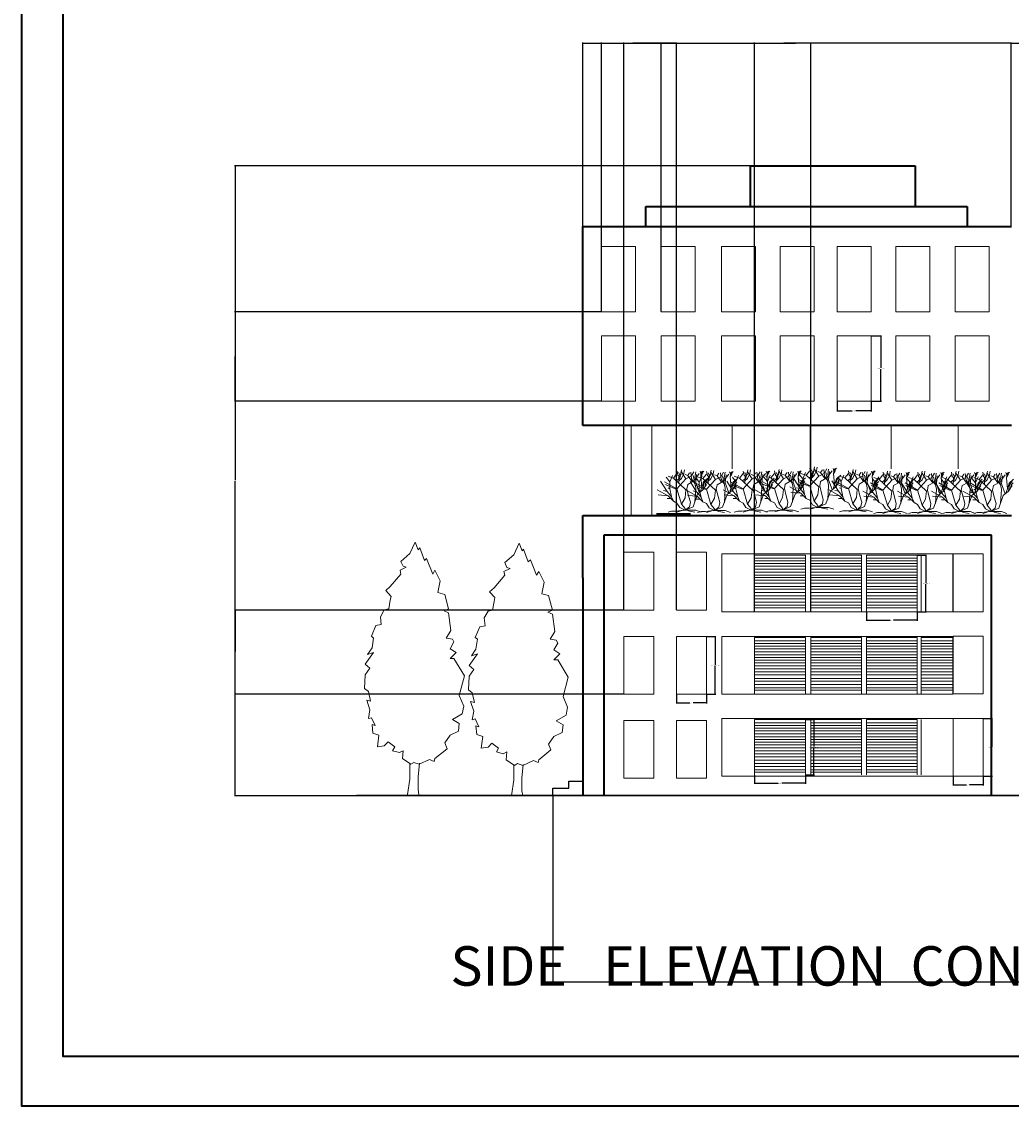
# Model space of a CAD drawing. Units: inches. Extents: x -279 to 364, y -385 to 335.
# Tile 1 of 9: x -279 to 7, y -385 to -72. Entities that reach past the tile are written whole.
import ezdxf

# ---------------------------------------------------------------- set-up
doc = ezdxf.new("R2010")
doc.units = ezdxf.units.IN
doc.header["$MEASUREMENT"] = 0
for name, color, linetype, lineweight in [('A-ANNO-DIMS', 2, 'Continuous', 18), ('A-ANNO-TEXT', 7, 'Continuous', 25), ('A-ANNO-TTLB', 7, 'Continuous', 35), ('A-FLOR-STRS', 7, 'Continuous', 25), ('A-GLAZ', 4, 'Continuous', 18), ('A-GLAZ-CURT', 4, 'Continuous', 18), ('A-ROOF', 7, 'Continuous', 35), ('A-WALL', 7, 'Continuous', 35), ('A-WALL-LOUV', 8, 'Continuous', 13), ('C-TOPO', 32, 'Continuous', 30), ('L-PLNT', 94, 'Continuous', 13)]:
    doc.layers.add(name, color=color, linetype=linetype, lineweight=lineweight)
doc.styles.get("Standard").update_dxf_attribs({"font": 'arial.ttf'})
doc.dimstyles.get("Standard").update_dxf_attribs({"dimtxt": 0.18, "dimasz": 0.18, "dimexe": 0.18, "dimexo": 0.0625, "dimgap": 0.09, "dimtad": 0, "dimtih": 1, "dimtoh": 1, "dimdec": 4, "dimzin": 0, "dimdsep": 46, "dimtxsty": 'Standard', "dimcen": 0.09, "dimadec": 0, "dimazin": 0, "dimtfac": 1, "dimtdec": 4, "dimtofl": 0, "dimtmove": 0, "dimatfit": 3, "dimfxl": 1, "dimtolj": 1, "dimtzin": 0, "dimarcsym": 0})

# ---------------------------------------------------------------- blocks, each defined once
blk = doc.blocks.new('*U2')
for p, q in [((-16.8, 16.32), (-18.72, 18.72)), ((-14.88, 18.24), (-17.76, 19.2)), ((-16.8, 16.32), (-15.36, 19.68)), ((-14.88, 18.24), (-12.96, 20.64)), ((-8.16, 12), (-14.88, 18.24)), ((-13.325, 16.724), (-11.433, 18.289)), ((-12.96, 12.48), (-8.16, 17.76)), ((-12.471, 19.775), (-12.898, 22.044)), ((-11.677, 19.071), (-12.471, 19.775)), ((-11.28, 19.619), (-12.104, 21.184)), ((-12.043, 15.628), (-11.921, 18.836)), ((-11.982, 16.802), (-10.579, 18.054)), ((-11.921, 18.836), (-10.64, 20.401)), ((-11.433, 18.289), (-10.457, 22.749)), ((-10.579, 18.054), (-9.846, 19.697)), ((-8.16, 17.76), (-10.56, 21.6)), ((-9.48, 19.775), (-8.992, 22.592)), ((-7.2, 19.68), (-8.64, 20.16)), ((-8.16, 17.76), (-5.28, 19.2)), ((-7.2, 19.68), (-6.24, 21.12)), ((-4.8, 16.32), (-7.2, 19.68)), ((-5.086, 17.741), (-5.513, 21.34)), ((-5.28, 19.2), (-3.84, 21.6)), ((-3.377, 15.315), (-5.086, 17.819)), ((-2.88, 12.96), (-4.32, 19.68)), ((-3.84, 16.8), (-0.96, 20.64)), ((-3.377, 18.602), (-2.888, 21.575)), ((-2.766, 16.802), (-3.377, 18.602)), ((-2.88, 15.84), (-2.4, 20.16)), ((-0.508, 21.888), (-0.081, 20.558)), ((-0.203, 19.149), (0.102, 21.34)), ((0.346, 13.203), (-0.203, 19.149)), ((-0.142, 19.384), (0.59, 20.401)), ((-0.02, 20.01), (0.896, 21.105)), ((0.041, 20.714), (1.384, 22.044)), ((0.102, 21.34), (0.835, 21.888)), ((1.323, 16.254), (3.642, 18.289)), ((-17.76, 8.64), (-23.663, 11.961)), ((-18.24, 11.04), (-21.755, 16.655)), ((-12.96, 12.48), (-19.68, 16.32)), ((-13.92, 12.48), (-19.2, 14.88)), ((-16.8, 12.48), (-17.76, 12.96)), ((-16.8, 12.48), (-16.8, 16.32)), ((-15.84, 8.16), (-16.8, 12.48)), ((-12.96, 12.48), (-13.92, 12.48)), ((-10.56, 4.32), (-12.96, 12.48)), ((-8.64, 7.68), (-8.16, 12)), ((-7.68, 12.48), (-7.2, 14.88)), ((-6.72, 8.64), (-7.68, 12.48)), ((-7.2, 14.88), (-3.84, 16.8)), ((-3.36, 5.28), (-2.88, 12.96)), ((-0.96, 10.56), (-2.88, 15.84)), ((-1.92, 9.6), (0.96, 12)), ((-0.48, 10.8), (0.346, 13.203)), ((0.346, 13.203), (1.323, 16.254)), ((0.96, 12), (1.44, 15.36)), ((0.96, 12), (2.88, 14.88)), ((1.44, 15.36), (2.88, 17.28)), ((1.92, 13.44), (2.4, 15.36)), ((2.4, 15.36), (3.36, 16.32)), ((-17.76, 8.64), (-23.128, 9.222)), ((-18.24, 11.04), (-20.16, 11.52)), ((-15.84, 8.16), (-18.24, 11.04)), ((-16.32, 7.2), (-18.24, 7.2)), ((-14.88, 5.76), (-17.76, 8.64)), ((-14.88, 5.76), (-15.84, 8.16)), ((-10.56, 4.32), (-8.64, 7.68)), ((-5.76, 5.28), (-6.72, 8.64)), ((-4.32, 2.88), (-1.92, 9.6)), ((-15.84, 0.48), (-17.76, 0)), ((-13.44, 0.48), (-15.84, 0.48)), ((-12.96, 4.8), (-14.88, 5.76)), ((-9.6, 0.96), (-13.44, 0.48)), ((-11.52, 2.4), (-12.96, 4.8)), ((-9.6, 0.96), (-12.96, 0)), ((-8.64, 0.96), (-11.52, 2.4)), ((-8.64, 1.92), (-10.56, 4.32)), ((-9.6, 0.96), (-7.68, 0.96)), ((-8.64, 0.96), (-4.32, 2.88)), ((-8.64, 0.96), (-6.24, 2.88)), ((-8.64, 0.96), (-8.64, 1.92)), ((-8.64, 0.96), (-2.88, 0.96)), ((-7.68, 0.96), (-6.24, 0.48)), ((-6.24, 2.88), (-5.76, 5.28)), ((-6.24, 0.48), (-3.36, 0)), ((-2.88, 0.96), (0, 0))]:
    blk.add_line(p, q)
blk = doc.blocks.new('*U3')
blk.add_lwpolyline([(-2.754, 191.699), (-6.78, 182.851), (-13.682, 176.953), (-11.956, 173.266), (-9.656, 172.529), (-14.257, 170.317), (-13.682, 167.368), (-21.733, 157.783), (-25.184, 154.834), (-21.158, 150.41), (-21.733, 147.461), (-22.884, 140.825), (-26.334, 140.087), (-29.21, 134.926), (-28.635, 129.028), (-32.661, 128.291), (-36.111, 120.18), (-34.386, 118.706), (-35.536, 111.333), (-38.987, 106.171), (-34.386, 107.646), (-40.712, 98.798), (-37.261, 95.849), (-40.712, 90.688), (-41.287, 80.366), (-38.412, 78.154), (-36.686, 70.781), (-39.562, 71.518), (-37.261, 64.145), (-38.412, 57.509), (-36.111, 58.247), (-33.236, 52.348), (-35.536, 53.086), (-34.961, 46.45), (-30.36, 44.975), (-31.51, 36.128), (-26.334, 36.865), (-23.459, 39.814), (-18.283, 36.128), (-20.008, 33.178), (-14.832, 31.704), (-11.956, 33.178), (-12.531, 27.28), (-6.205, 22.856), (-3.905, 24.331), (0.121, 22.856), (8.173, 26.543), (11.624, 25.068), (12.199, 27.28), (21.4, 34.653), (19.675, 39.077), (23.701, 44.975), (30.027, 47.924), (30.602, 53.823), (25.426, 56.772), (32.903, 61.196), (34.053, 67.094), (30.602, 75.205), (34.628, 89.951), (26.576, 103.222), (23.701, 103.222), (28.302, 107.646), (23.701, 110.595), (26.576, 115.756), (25.426, 117.968), (20.825, 118.706), (24.276, 124.604), (22.551, 137.876), (19.1, 139.35), (22.551, 140.825), (19.675, 151.884), (14.499, 153.359), (16.224, 162.207), (12.199, 170.317), (10.473, 167.368), (5.872, 179.165), (4.147, 177.69), (0.696, 187.275), (-0.454, 185.8)], close=True)
for points in [[(-6.813, 23.669), (-6.813, 11.669), (-8.627, 0)], [(0.387, 23.669), (-0.576, 13.271), (-0.576, 3.686), (0, 0)]]:
    blk.add_lwpolyline(points)
blk = doc.blocks.new('WIN-TOWER-SIDE')
for p, q in [((9.82, 18.84), (0, 18.84)), ((0, 18.84), (0, 17.44)), ((9.82, 0), (9.82, 18.84)), ((0, 17.44), (0, 0)), ((0, 0), (9.82, 0))]:
    blk.add_line(p, q)
blk = doc.blocks.new('WIN-SIDE-SINGLE')
for p, q in [((8.72, 16.72), (0, 16.72)), ((0, 16.72), (0, 15.47)), ((8.72, 0), (8.72, 16.72)), ((0, 15.47), (0, 0)), ((0, 0), (8.72, 0))]:
    blk.add_line(p, q)
blk = doc.blocks.new('LOUVER-SIDE-SILL')
for p, q in [((0, 15.99), (14.71, 15.99)), ((0, 15.99), (0, 0)), ((14.71, 15.99), (14.71, 0)), ((0, 15.1), (14.71, 15.1)), ((0, 14.31), (14.71, 14.31)), ((0, 13.56), (14.71, 13.56)), ((0, 12.75), (14.71, 12.75)), ((0, 11.88), (14.71, 11.88)), ((0, 11.04), (14.71, 11.04)), ((0, 10.21), (14.71, 10.21)), ((0, 9.5), (14.71, 9.5)), ((0, 8.71), (14.71, 8.71)), ((0, 7.84), (14.71, 7.84)), ((0, 6.96), (14.71, 6.96)), ((0, 6.12), (14.71, 6.12)), ((0, 5.22), (14.71, 5.22)), ((0, 4.22), (14.71, 4.22)), ((0, 3.35), (14.71, 3.35)), ((0, 2.4), (14.71, 2.4)), ((0, 1.49), (14.71, 1.49)), ((0, 0.76), (14.71, 0.76))]:
    blk.add_line(p, q)
blk = doc.blocks.new('LOUVER-SIDE-FIELD')
for p, q in [((0, 16.37), (14.71, 16.37)), ((0, 16.37), (0, 0)), ((14.71, 16.37), (14.71, 0)), ((0, 15.48), (14.71, 15.48)), ((0, 14.69), (14.71, 14.69)), ((0, 13.94), (14.71, 13.94)), ((0, 13.13), (14.71, 13.13)), ((0, 12.27), (14.71, 12.27)), ((0, 11.42), (14.71, 11.42)), ((0, 10.6), (14.71, 10.6)), ((0, 9.88), (14.71, 9.88)), ((0, 9.09), (14.71, 9.09)), ((0, 8.22), (14.71, 8.22)), ((0, 7.34), (14.71, 7.34)), ((0, 6.5), (14.71, 6.5)), ((0, 5.6), (14.71, 5.6)), ((0, 4.6), (14.71, 4.6)), ((0, 3.74), (14.71, 3.74)), ((0, 2.78), (14.71, 2.78)), ((0, 1.88), (14.71, 1.88)), ((0, 1.14), (14.71, 1.14))]:
    blk.add_line(p, q)
blk = doc.blocks.new('WIN-SIDE-END')
for p, q in [((0, 16.72), (8.68, 16.72)), ((0, 16.54), (0, 15.3)), ((8.68, 16.72), (8.68, 0)), ((0, 15.3), (0, 0)), ((8.68, 0), (0, 0))]:
    blk.add_line(p, q)
blk = doc.blocks.new('*D36')
at = {"layer": 'A-ANNO-DIMS', "color": 0, "lineweight": -2, "transparency": 16777216}
for p, q in [((-33.52, -162.47), (-30.58, -162.47)), ((-30.76, -162.65), (-30.76, -171.71)), ((-30.76, -181.13), (-30.76, -172.07)), ((-33.52, -181.31), (-30.58, -181.31))]:
    blk.add_line(p, q, dxfattribs=at)
at = {"layer": 'A-ANNO-DIMS', "color": 0, "transparency": 16777216}
for points in [[(-30.79, -162.65), (-30.73, -162.65), (-30.76, -162.47)], [(-30.79, -181.13), (-30.73, -181.13), (-30.76, -181.31)]]:
    blk.add_solid(points, dxfattribs=at)
at = {"layer": 'Defpoints', "color": 0, "transparency": 16777216}
for p in [(-33.58, -162.47), (-30.76, -162.47), (-33.58, -181.31)]:
    blk.add_point(p, dxfattribs=at)
at = {"layer": 'A-ANNO-DIMS', "color": 0, "transparency": 16777216, "insert": (-30.76, -171.89), "char_height": 0.18, "attachment_point": 5}
blk.add_mtext('\\A1;TOWER SASH 19 TYP.', dxfattribs=at)
blk = doc.blocks.new('*D37')
at = {"layer": 'A-ANNO-DIMS', "color": 0, "lineweight": -2, "transparency": 16777216}
for p, q in [((-43.41, -181.37), (-43.41, -184.32)), ((-33.58, -181.37), (-33.58, -184.32)), ((-43.23, -184.14), (-39.01, -184.14)), ((-33.76, -184.14), (-37.98, -184.14))]:
    blk.add_line(p, q, dxfattribs=at)
at = {"layer": 'A-ANNO-DIMS', "color": 0, "transparency": 16777216}
for points in [[(-43.23, -184.11), (-43.23, -184.17), (-43.41, -184.14)], [(-33.76, -184.11), (-33.76, -184.17), (-33.58, -184.14)]]:
    blk.add_solid(points, dxfattribs=at)
at = {"layer": 'Defpoints', "color": 0, "transparency": 16777216}
for p in [(-43.41, -181.31), (-33.58, -181.31), (-33.58, -184.14)]:
    blk.add_point(p, dxfattribs=at)
at = {"layer": 'A-ANNO-DIMS', "color": 0, "transparency": 16777216, "insert": (-38.49, -184.14), "char_height": 0.18, "attachment_point": 5}
blk.add_mtext('\\A1;10 TYP.', dxfattribs=at)
blk = doc.blocks.new('*D38')
at = {"layer": 'A-ANNO-DIMS', "color": 0, "lineweight": -2, "transparency": 16777216}
for p, q in [((-81.07, -249.35), (-78.44, -249.35)), ((-78.62, -249.53), (-78.62, -257.53)), ((-78.62, -265.89), (-78.62, -257.9)), ((-81.07, -266.07), (-78.44, -266.07))]:
    blk.add_line(p, q, dxfattribs=at)
at = {"layer": 'A-ANNO-DIMS', "color": 0, "transparency": 16777216}
for points in [[(-78.65, -249.53), (-78.59, -249.53), (-78.62, -249.35)], [(-78.65, -265.89), (-78.59, -265.89), (-78.62, -266.07)]]:
    blk.add_solid(points, dxfattribs=at)
at = {"layer": 'Defpoints', "color": 0, "transparency": 16777216}
for p in [(-81.13, -249.35), (-78.62, -249.35), (-81.13, -266.07)]:
    blk.add_point(p, dxfattribs=at)
at = {"layer": 'A-ANNO-DIMS', "color": 0, "transparency": 16777216, "insert": (-78.62, -257.71), "char_height": 0.18, "attachment_point": 5}
blk.add_mtext('\\A1;SINGLE SASH 17 TYP.', dxfattribs=at)
blk = doc.blocks.new('*D39')
at = {"layer": 'A-ANNO-DIMS', "color": 0, "lineweight": -2, "transparency": 16777216}
for p, q in [((-89.84, -266.13), (-89.84, -268.76)), ((-81.13, -266.13), (-81.13, -268.76)), ((-89.66, -268.58), (-85.95, -268.58)), ((-81.31, -268.58), (-85.03, -268.58))]:
    blk.add_line(p, q, dxfattribs=at)
at = {"layer": 'A-ANNO-DIMS', "color": 0, "transparency": 16777216}
for points in [[(-89.66, -268.55), (-89.66, -268.61), (-89.84, -268.58)], [(-81.31, -268.55), (-81.31, -268.61), (-81.13, -268.58)]]:
    blk.add_solid(points, dxfattribs=at)
at = {"layer": 'Defpoints', "color": 0, "transparency": 16777216}
for p in [(-89.84, -266.07), (-81.13, -266.07), (-81.13, -268.58)]:
    blk.add_point(p, dxfattribs=at)
at = {"layer": 'A-ANNO-DIMS', "color": 0, "transparency": 16777216, "insert": (-85.49, -268.58), "char_height": 0.18, "attachment_point": 5}
blk.add_mtext('\\A1;9 TYP.', dxfattribs=at)
blk = doc.blocks.new('*D48')
at = {"layer": 'A-ANNO-DIMS', "color": 0, "lineweight": -2, "transparency": 16777216}
for p, q in [((-20.16, -225.83), (-17.58, -225.83)), ((-17.76, -226.01), (-17.76, -233.84)), ((-17.76, -242.03), (-17.76, -234.2)), ((-20.16, -242.21), (-17.58, -242.21))]:
    blk.add_line(p, q, dxfattribs=at)
at = {"layer": 'A-ANNO-DIMS', "color": 0, "transparency": 16777216}
for points in [[(-17.79, -226.01), (-17.73, -226.01), (-17.76, -225.83)], [(-17.79, -242.03), (-17.73, -242.03), (-17.76, -242.21)]]:
    blk.add_solid(points, dxfattribs=at)
at = {"layer": 'Defpoints', "color": 0, "transparency": 16777216}
for p in [(-20.22, -225.83), (-17.76, -225.83), (-20.22, -242.21)]:
    blk.add_point(p, dxfattribs=at)
at = {"layer": 'A-ANNO-DIMS', "color": 0, "transparency": 16777216, "insert": (-17.76, -234.02), "char_height": 0.18, "attachment_point": 5}
blk.add_mtext('\\A1;FIELD LOUVER 16 TYP.', dxfattribs=at)
blk = doc.blocks.new('*D49')
at = {"layer": 'A-ANNO-DIMS', "color": 0, "lineweight": -2, "transparency": 16777216}
for p, q in [((-34.93, -242.27), (-34.93, -244.84)), ((-20.22, -242.27), (-20.22, -244.84)), ((-34.75, -244.66), (-28.09, -244.66)), ((-20.4, -244.66), (-27.06, -244.66))]:
    blk.add_line(p, q, dxfattribs=at)
at = {"layer": 'A-ANNO-DIMS', "color": 0, "transparency": 16777216}
for points in [[(-34.75, -244.63), (-34.75, -244.69), (-34.93, -244.66)], [(-20.4, -244.63), (-20.4, -244.69), (-20.22, -244.66)]]:
    blk.add_solid(points, dxfattribs=at)
at = {"layer": 'Defpoints', "color": 0, "transparency": 16777216}
for p in [(-34.93, -242.21), (-20.22, -242.21), (-20.22, -244.66)]:
    blk.add_point(p, dxfattribs=at)
at = {"layer": 'A-ANNO-DIMS', "color": 0, "transparency": 16777216, "insert": (-27.57, -244.66), "char_height": 0.18, "attachment_point": 5}
blk.add_mtext('\\A1;15 TYP.', dxfattribs=at)
blk = doc.blocks.new('*D50')
at = {"layer": 'A-ANNO-DIMS', "color": 0, "lineweight": -2, "transparency": 16777216}
for p, q in [((-52.49, -273.41), (-49.98, -273.41)), ((-50.16, -273.59), (-50.16, -281.22)), ((-50.16, -289.22), (-50.16, -281.59)), ((-52.49, -289.4), (-49.98, -289.4))]:
    blk.add_line(p, q, dxfattribs=at)
at = {"layer": 'A-ANNO-DIMS', "color": 0, "transparency": 16777216}
for points in [[(-50.19, -273.59), (-50.13, -273.59), (-50.16, -273.41)], [(-50.19, -289.22), (-50.13, -289.22), (-50.16, -289.4)]]:
    blk.add_solid(points, dxfattribs=at)
at = {"layer": 'Defpoints', "color": 0, "transparency": 16777216}
for p in [(-52.55, -273.41), (-50.16, -273.41), (-52.55, -289.4)]:
    blk.add_point(p, dxfattribs=at)
at = {"layer": 'A-ANNO-DIMS', "color": 0, "transparency": 16777216, "insert": (-50.16, -281.4), "char_height": 0.18, "attachment_point": 5}
blk.add_mtext('\\A1;SILL LOUVER 16 TYP.', dxfattribs=at)
blk = doc.blocks.new('*D51')
at = {"layer": 'A-ANNO-DIMS', "color": 0, "lineweight": -2, "transparency": 16777216}
for p, q in [((-67.26, -289.46), (-67.26, -291.98)), ((-52.55, -289.46), (-52.55, -291.98)), ((-67.08, -291.8), (-60.43, -291.8)), ((-52.73, -291.8), (-59.39, -291.8))]:
    blk.add_line(p, q, dxfattribs=at)
at = {"layer": 'A-ANNO-DIMS', "color": 0, "transparency": 16777216}
for points in [[(-67.08, -291.77), (-67.08, -291.83), (-67.26, -291.8)], [(-52.73, -291.77), (-52.73, -291.83), (-52.55, -291.8)]]:
    blk.add_solid(points, dxfattribs=at)
at = {"layer": 'Defpoints', "color": 0, "transparency": 16777216}
for p in [(-67.26, -289.4), (-52.55, -289.4), (-52.55, -291.8)]:
    blk.add_point(p, dxfattribs=at)
at = {"layer": 'A-ANNO-DIMS', "color": 0, "transparency": 16777216, "insert": (-59.91, -291.8), "char_height": 0.18, "attachment_point": 5}
blk.add_mtext('\\A1;15 TYP.', dxfattribs=at)
blk = doc.blocks.new('*D60')
at = {"layer": 'A-ANNO-DIMS', "color": 0, "lineweight": -2, "transparency": 16777216}
for p, q in [((-1.13, -273.06), (1.5, -273.06)), ((1.32, -273.24), (1.32, -281.24)), ((1.32, -289.6), (1.32, -281.61)), ((-1.13, -289.78), (1.5, -289.78))]:
    blk.add_line(p, q, dxfattribs=at)
at = {"layer": 'A-ANNO-DIMS', "color": 0, "transparency": 16777216}
for points in [[(1.29, -273.24), (1.35, -273.24), (1.32, -273.06)], [(1.29, -289.6), (1.35, -289.6), (1.32, -289.78)]]:
    blk.add_solid(points, dxfattribs=at)
at = {"layer": 'Defpoints', "color": 0, "transparency": 16777216}
for p in [(-1.19, -273.06), (1.32, -273.06), (-1.19, -289.78)]:
    blk.add_point(p, dxfattribs=at)
at = {"layer": 'A-ANNO-DIMS', "color": 0, "transparency": 16777216, "insert": (1.32, -281.42), "char_height": 0.18, "attachment_point": 5}
blk.add_mtext('\\A1;END SASH 17 TYP.', dxfattribs=at)
blk = doc.blocks.new('*D61')
at = {"layer": 'A-ANNO-DIMS', "color": 0, "lineweight": -2, "transparency": 16777216}
for p, q in [((-9.87, -289.84), (-9.87, -292.47)), ((-1.19, -289.84), (-1.19, -292.47)), ((-9.69, -292.29), (-5.99, -292.29)), ((-1.37, -292.29), (-5.07, -292.29))]:
    blk.add_line(p, q, dxfattribs=at)
at = {"layer": 'A-ANNO-DIMS', "color": 0, "transparency": 16777216}
for points in [[(-9.69, -292.26), (-9.69, -292.32), (-9.87, -292.29)], [(-1.37, -292.26), (-1.37, -292.32), (-1.19, -292.29)]]:
    blk.add_solid(points, dxfattribs=at)
at = {"layer": 'Defpoints', "color": 0, "transparency": 16777216}
for p in [(-9.87, -289.78), (-1.19, -289.78), (-1.19, -292.29)]:
    blk.add_point(p, dxfattribs=at)
at = {"layer": 'A-ANNO-DIMS', "color": 0, "transparency": 16777216, "insert": (-5.53, -292.29), "char_height": 0.18, "attachment_point": 5}
blk.add_mtext('\\A1;9 TYP.', dxfattribs=at)
blk = doc.blocks.new('*D97')
at = {"layer": 'A-ANNO-DIMS', "color": 0, "lineweight": -2, "transparency": 16777216}
for p, q in [((243.83, -291), (243.83, -349.37)), ((-125.57, -295.46), (-125.57, -349.37)), ((-125.39, -349.19), (58.74, -349.19)), ((243.65, -349.19), (59.52, -349.19))]:
    blk.add_line(p, q, dxfattribs=at)
at = {"layer": 'A-ANNO-DIMS', "color": 0, "transparency": 16777216}
for points in [[(-125.39, -349.16), (-125.39, -349.22), (-125.57, -349.19)], [(243.65, -349.16), (243.65, -349.22), (243.83, -349.19)]]:
    blk.add_solid(points, dxfattribs=at)
at = {"layer": 'Defpoints', "color": 0, "transparency": 16777216}
for p in [(243.83, -290.94), (-125.57, -295.4), (243.83, -349.19)]:
    blk.add_point(p, dxfattribs=at)
at = {"layer": 'A-ANNO-DIMS', "color": 0, "transparency": 16777216, "insert": (59.13, -349.19), "char_height": 0.18, "attachment_point": 5}
blk.add_mtext('\\A1;369.4', dxfattribs=at)
blk = doc.blocks.new('*D98')
at = {"layer": 'A-ANNO-DIMS', "color": 0, "lineweight": -2, "transparency": 16777216}
for p, q in [((-68.51, -113.25), (-217.68, -113.25)), ((-217.5, -113.43), (-217.5, -204.14)), ((-217.5, -295.22), (-217.5, -204.5)), ((-117.04, -295.4), (-217.68, -295.4))]:
    blk.add_line(p, q, dxfattribs=at)
at = {"layer": 'A-ANNO-DIMS', "color": 0, "transparency": 16777216}
for points in [[(-217.53, -113.43), (-217.47, -113.43), (-217.5, -113.25)], [(-217.53, -295.22), (-217.47, -295.22), (-217.5, -295.4)]]:
    blk.add_solid(points, dxfattribs=at)
at = {"layer": 'Defpoints', "color": 0, "transparency": 16777216}
for p in [(-217.5, -113.25), (-68.45, -113.25), (-116.98, -295.4)]:
    blk.add_point(p, dxfattribs=at)
at = {"layer": 'A-ANNO-DIMS', "color": 0, "transparency": 16777216, "insert": (-217.5, -204.32), "char_height": 0.18, "attachment_point": 5}
blk.add_mtext('\\A1;182.15', dxfattribs=at)
blk = doc.blocks.new('*D99')
at = {"layer": 'A-ANNO-DIMS', "color": 0, "lineweight": -2, "transparency": 16777216}
for p, q in [((-116.98, -130.8), (-116.98, -77.65)), ((-116.8, -77.83), (-55.46, -77.83)), ((6.78, -77.83), (-54.56, -77.83)), ((6.96, -130.63), (6.96, -77.65))]:
    blk.add_line(p, q, dxfattribs=at)
at = {"layer": 'A-ANNO-DIMS', "color": 0, "transparency": 16777216}
for points in [[(-116.8, -77.8), (-116.8, -77.86), (-116.98, -77.83)], [(6.78, -77.8), (6.78, -77.86), (6.96, -77.83)]]:
    blk.add_solid(points, dxfattribs=at)
at = {"layer": 'Defpoints', "color": 0, "transparency": 16777216}
for p in [(6.96, -77.83), (-116.98, -130.86), (6.96, -130.69)]:
    blk.add_point(p, dxfattribs=at)
at = {"layer": 'A-ANNO-DIMS', "color": 0, "transparency": 16777216, "insert": (-55.01, -77.83), "char_height": 0.18, "attachment_point": 5}
blk.add_mtext('\\A1;123.94', dxfattribs=at)
blk = doc.blocks.new('*D100')
at = {"layer": 'A-ANNO-DIMS', "color": 0, "lineweight": -2, "transparency": 16777216}
for p, q in [((6.96, -130.63), (6.96, -77.65)), ((7.14, -77.83), (60.2, -77.83)), ((114.17, -77.83), (61.11, -77.83)), ((114.35, -130.65), (114.35, -77.65))]:
    blk.add_line(p, q, dxfattribs=at)
at = {"layer": 'A-ANNO-DIMS', "color": 0, "transparency": 16777216}
for points in [[(7.14, -77.8), (7.14, -77.86), (6.96, -77.83)], [(114.17, -77.8), (114.17, -77.86), (114.35, -77.83)]]:
    blk.add_solid(points, dxfattribs=at)
at = {"layer": 'Defpoints', "color": 0, "transparency": 16777216}
for p in [(114.35, -77.83), (6.96, -130.69), (114.35, -130.71)]:
    blk.add_point(p, dxfattribs=at)
at = {"layer": 'A-ANNO-DIMS', "color": 0, "transparency": 16777216, "insert": (60.65, -77.83), "char_height": 0.18, "attachment_point": 5}
blk.add_mtext('\\A1;107.38', dxfattribs=at)
blk = doc.blocks.new('*D105')
at = {"layer": 'A-ANNO-DIMS', "color": 0, "lineweight": -2, "transparency": 16777216}
for p, q in [((-111.51, -155.43), (-111.51, -77.65)), ((-111.33, -77.83), (-103.35, -77.83)), ((-94.47, -77.83), (-102.45, -77.83)), ((-94.29, -155.43), (-94.29, -77.65))]:
    blk.add_line(p, q, dxfattribs=at)
at = {"layer": 'A-ANNO-DIMS', "color": 0, "transparency": 16777216}
for points in [[(-111.33, -77.8), (-111.33, -77.86), (-111.51, -77.83)], [(-94.47, -77.8), (-94.47, -77.86), (-94.29, -77.83)]]:
    blk.add_solid(points, dxfattribs=at)
at = {"layer": 'Defpoints', "color": 0, "transparency": 16777216}
for p in [(-94.29, -77.83), (-111.51, -155.49), (-94.29, -155.49)]:
    blk.add_point(p, dxfattribs=at)
at = {"layer": 'A-ANNO-DIMS', "color": 0, "transparency": 16777216, "insert": (-102.9, -77.83), "char_height": 0.18, "attachment_point": 5}
blk.add_mtext('\\A1;17.212', dxfattribs=at)
blk = doc.blocks.new('*D106')
at = {"layer": 'A-ANNO-DIMS', "color": 0, "lineweight": -2, "transparency": 16777216}
for p, q in [((-111.57, -155.49), (-217.68, -155.49)), ((-217.5, -155.67), (-217.5, -168.22)), ((-217.5, -181.13), (-217.5, -168.58)), ((-111.57, -181.31), (-217.68, -181.31))]:
    blk.add_line(p, q, dxfattribs=at)
at = {"layer": 'A-ANNO-DIMS', "color": 0, "transparency": 16777216}
for points in [[(-217.53, -155.67), (-217.47, -155.67), (-217.5, -155.49)], [(-217.53, -181.13), (-217.47, -181.13), (-217.5, -181.31)]]:
    blk.add_solid(points, dxfattribs=at)
at = {"layer": 'Defpoints', "color": 0, "transparency": 16777216}
for p in [(-217.5, -155.49), (-111.51, -155.49), (-111.51, -181.31)]:
    blk.add_point(p, dxfattribs=at)
at = {"layer": 'A-ANNO-DIMS', "color": 0, "transparency": 16777216, "insert": (-217.5, -168.4), "char_height": 0.18, "attachment_point": 5}
blk.add_mtext('\\A1;25.824', dxfattribs=at)
blk = doc.blocks.new('*D107')
at = {"layer": 'A-ANNO-DIMS', "color": 0, "lineweight": -2, "transparency": 16777216}
for p, q in [((-105.11, -241.66), (-105.11, -77.65)), ((-104.93, -77.83), (-97.86, -77.83)), ((-90.02, -77.83), (-97.09, -77.83)), ((-89.84, -241.66), (-89.84, -77.65))]:
    blk.add_line(p, q, dxfattribs=at)
at = {"layer": 'A-ANNO-DIMS', "color": 0, "transparency": 16777216}
for points in [[(-104.93, -77.8), (-104.93, -77.86), (-105.11, -77.83)], [(-90.02, -77.8), (-90.02, -77.86), (-89.84, -77.83)]]:
    blk.add_solid(points, dxfattribs=at)
at = {"layer": 'Defpoints', "color": 0, "transparency": 16777216}
for p in [(-89.84, -77.83), (-105.11, -241.72), (-89.84, -241.72)]:
    blk.add_point(p, dxfattribs=at)
at = {"layer": 'A-ANNO-DIMS', "color": 0, "transparency": 16777216, "insert": (-97.48, -77.83), "char_height": 0.18, "attachment_point": 5}
blk.add_mtext('\\A1;15.27', dxfattribs=at)
blk = doc.blocks.new('*D108')
at = {"layer": 'A-ANNO-DIMS', "color": 0, "lineweight": -2, "transparency": 16777216}
for p, q in [((-105.18, -241.72), (-217.68, -241.72)), ((-217.5, -241.9), (-217.5, -253.71)), ((-217.5, -265.89), (-217.5, -254.08)), ((-105.18, -266.07), (-217.68, -266.07))]:
    blk.add_line(p, q, dxfattribs=at)
at = {"layer": 'A-ANNO-DIMS', "color": 0, "transparency": 16777216}
for points in [[(-217.53, -241.9), (-217.47, -241.9), (-217.5, -241.72)], [(-217.53, -265.89), (-217.47, -265.89), (-217.5, -266.07)]]:
    blk.add_solid(points, dxfattribs=at)
at = {"layer": 'Defpoints', "color": 0, "transparency": 16777216}
for p in [(-105.11, -241.72), (-217.5, -266.07), (-105.11, -266.07)]:
    blk.add_point(p, dxfattribs=at)
at = {"layer": 'A-ANNO-DIMS', "color": 0, "transparency": 16777216, "insert": (-217.5, -253.9), "char_height": 0.18, "attachment_point": 5}
blk.add_mtext('\\A1;24.35', dxfattribs=at)
blk = doc.blocks.new('*D109')
at = {"layer": 'A-ANNO-DIMS', "color": 0, "lineweight": -2, "transparency": 16777216}
for p, q in [((-67.26, -242.14), (-67.26, -77.65)), ((-67.08, -77.83), (-59.53, -77.83)), ((-51.21, -77.83), (-58.76, -77.83)), ((-51.03, -242.14), (-51.03, -77.65))]:
    blk.add_line(p, q, dxfattribs=at)
at = {"layer": 'A-ANNO-DIMS', "color": 0, "transparency": 16777216}
for points in [[(-67.08, -77.8), (-67.08, -77.86), (-67.26, -77.83)], [(-51.21, -77.8), (-51.21, -77.86), (-51.03, -77.83)]]:
    blk.add_solid(points, dxfattribs=at)
at = {"layer": 'Defpoints', "color": 0, "transparency": 16777216}
for p in [(-51.03, -77.83), (-67.26, -242.21), (-51.03, -242.21)]:
    blk.add_point(p, dxfattribs=at)
at = {"layer": 'A-ANNO-DIMS', "color": 0, "transparency": 16777216, "insert": (-59.15, -77.83), "char_height": 0.18, "attachment_point": 5}
blk.add_mtext('\\A1;16.23', dxfattribs=at)

msp = doc.modelspace()

# ---------------------------------------------------------------- linework, layer by layer
at = {"layer": 'A-ANNO-TTLB'}
for points in [[(-279.2289, 334.6468), (364.0508, 334.6468), (364.0508, -385.2219), (-279.2289, -385.2219)], [(-267.2403, 317.5778), (348.1051, 317.5778), (348.1051, -370.8321), (-267.2403, -370.8321)]]:
    msp.add_lwpolyline(points, close=True, dxfattribs=at)
at = {"layer": 'A-FLOR-STRS'}
for p, q in [((-120.9936, -293.218), (-120.9936, -291.2398)), ((-120.9936, -291.2398), (-116.9812, -291.2398)), ((-125.5669, -295.3951), (-125.5669, -293.218)), ((-125.5669, -293.218), (-120.9936, -293.218))]:
    msp.add_line(p, q, dxfattribs=at)
at = {"layer": 'A-GLAZ-CURT'}
for p, q in [((-102.9958, -188.3649), (-102.9958, -214.3585)), ((-97.0123, -188.3649), (-97.0123, -214.3585)), ((-73.7047, -188.3649), (-73.7047, -200.8785)), ((-51.1657, -188.3649), (-51.1657, -201.1299)), ((-27.7599, -188.3649), (-27.7599, -200.8785)), ((-8.3994, -188.3649), (-8.3994, -200.8785))]:
    msp.add_line(p, q, dxfattribs=at)
at = {"layer": 'A-ROOF'}
for p, q in [((-68.4486, -125.0697), (-68.4486, -113.2485)), ((-68.4486, -113.2485), (-20.8253, -113.2485)), ((-20.8253, -113.2485), (-20.8253, -125.0697)), ((-98.7002, -130.861), (-98.7002, -125.0697)), ((-98.7002, -125.0697), (-5.7456, -125.0697)), ((-5.7456, -125.0697), (-5.7456, -130.861))]:
    msp.add_line(p, q, dxfattribs=at)
at = {"layer": 'A-WALL'}
for p, q in [((-116.9812, -188.3649), (-116.9812, -130.861)), ((-116.9812, -130.861), (7.0091, -130.861)), ((7.0091, -188.3649), (-116.9812, -188.3649)), ((-116.9812, -232.4219), (-116.9812, -214.3585)), ((-116.9812, -214.3585), (7.0091, -214.3585)), ((-85.816, -214.0225), (-95.6453, -214.0225)), ((1.2469, -220.0327), (-110.8334, -220.0327)), ((-110.8334, -220.0327), (-110.8334, -295.3951)), ((1.2469, -295.3951), (1.2469, -220.0327)), ((-116.9812, -232.4219), (-116.9812, -295.3951))]:
    msp.add_line(p, q, dxfattribs=at)
at = {"layer": 'A-WALL-LOUV'}
for p, q in [((-76.7709, -225.4892), (-9.9162, -225.4892)), ((-76.7709, -225.4892), (-76.7709, -242.2074)), ((-9.9162, -225.4892), (-9.9162, -242.2074)), ((-19.0721, -225.8338), (-19.0721, -242.2074)), ((-76.7709, -242.2074), (-9.9162, -242.2074)), ((-81.1647, -249.6979), (-81.1294, -249.6979)), ((-81.1647, -250.5893), (-81.1294, -250.5893)), ((-76.7709, -249.3534), (-9.9162, -249.3534)), ((-76.7709, -249.3534), (-76.7709, -266.0715)), ((-19.0721, -249.6979), (-19.0721, -266.0715)), ((-19.0721, -249.6979), (-9.9162, -249.6979)), ((-19.0721, -250.5893), (-9.9162, -250.5893)), ((-9.9162, -249.3534), (-9.9162, -266.0715)), ((-81.1647, -251.3825), (-81.1294, -251.3825)), ((-81.1647, -252.1329), (-81.1294, -252.1329)), ((-81.1647, -252.9395), (-81.1294, -252.9395)), ((-81.1647, -253.8056), (-81.1294, -253.8056)), ((-19.0721, -251.3825), (-9.9162, -251.3825)), ((-19.0721, -252.1329), (-9.9162, -252.1329)), ((-19.0721, -252.9395), (-9.9162, -252.9395)), ((-19.0721, -253.8056), (-9.9162, -253.8056)), ((-81.1647, -254.6497), (-81.1294, -254.6497)), ((-81.1647, -255.4752), (-81.1294, -255.4752)), ((-81.1647, -256.188), (-81.1294, -256.188)), ((-81.1647, -256.9815), (-81.1294, -256.9815)), ((-19.0721, -254.6497), (-9.9162, -254.6497)), ((-19.0721, -255.4752), (-9.9162, -255.4752)), ((-19.0721, -256.188), (-9.9162, -256.188)), ((-19.0721, -256.9815), (-9.9162, -256.9815)), ((-81.1647, -257.8476), (-81.1294, -257.8476)), ((-81.1647, -258.7293), (-81.1294, -258.7293)), ((-81.1647, -259.5735), (-81.1294, -259.5735)), ((-19.0721, -257.8476), (-9.9162, -257.8476)), ((-19.0721, -258.7293), (-9.9162, -258.7293)), ((-19.0721, -259.5735), (-9.9162, -259.5735)), ((-81.1647, -260.474), (-81.1294, -260.474)), ((-81.1647, -261.4682), (-81.1294, -261.4682)), ((-81.1647, -262.3351), (-81.1294, -262.3351)), ((-81.1647, -263.2919), (-81.1294, -263.2919)), ((-19.0721, -260.474), (-9.9162, -260.474)), ((-19.0721, -261.4682), (-9.9162, -261.4682)), ((-19.0721, -262.3351), (-9.9162, -262.3351)), ((-19.0721, -263.2919), (-9.9162, -263.2919)), ((-81.1647, -264.1965), (-81.1294, -264.1965)), ((-81.1647, -264.9281), (-81.1294, -264.9281)), ((-81.1294, -265.6886), (-81.1647, -265.6886)), ((-76.7709, -266.0715), (-9.9162, -266.0715)), ((-19.0721, -264.1965), (-9.9162, -264.1965)), ((-19.0721, -264.9281), (-9.9162, -264.9281)), ((-76.7709, -273.0633), (-9.9162, -273.0633)), ((-76.7709, -273.0633), (-76.7709, -289.7814)), ((-19.0721, -273.4078), (-19.0721, -289.3986)), ((-76.7709, -289.7814), (-9.8683, -289.7814))]:
    msp.add_line(p, q, dxfattribs=at)
at = {"layer": 'C-TOPO'}
for q in [(-182.3634, -295.3951), (195.2296, -295.3951)]:
    msp.add_line((-116.9812, -295.3951), q, dxfattribs=at)

# ---------------------------------------------------------------- block references
at = {"layer": 'A-GLAZ'}
for name, p in [('WIN-TOWER-SIDE', (-111.506, -155.4878)), ('WIN-TOWER-SIDE', (-94.294, -155.4878)), ('WIN-TOWER-SIDE', (-76.8325, -155.4878)), ('WIN-TOWER-SIDE', (-59.8699, -155.4878)), ('WIN-TOWER-SIDE', (-43.4062, -155.4878)), ('WIN-TOWER-SIDE', (-26.4436, -155.4878)), ('WIN-TOWER-SIDE', (-9.2315, -155.4878)), ('WIN-TOWER-SIDE', (-111.506, -181.312)), ('WIN-TOWER-SIDE', (-94.294, -181.312)), ('WIN-TOWER-SIDE', (-76.8325, -181.312)), ('WIN-TOWER-SIDE', (-59.8699, -181.312)), ('WIN-TOWER-SIDE', (-43.4062, -181.312)), ('WIN-TOWER-SIDE', (-26.4436, -181.312)), ('WIN-TOWER-SIDE', (-9.2315, -181.312)), ('WIN-SIDE-SINGLE', (-105.115, -241.721)), ('WIN-SIDE-SINGLE', (-89.8445, -241.721)), ('WIN-SIDE-END', (-9.868, -242.2277)), ('WIN-SIDE-SINGLE', (-105.115, -266.0716)), ('WIN-SIDE-SINGLE', (-89.8445, -266.0716)), ('WIN-SIDE-END', (-9.868, -265.9701)), ('WIN-SIDE-SINGLE', (-105.115, -290.382)), ('WIN-SIDE-SINGLE', (-89.8445, -290.382)), ('WIN-SIDE-END', (-9.868, -289.781))]:
    msp.add_blockref(name, p, dxfattribs=at)
at = {"layer": 'A-WALL-LOUV'}
for name, p in [('LOUVER-SIDE-FIELD', (-67.262, -242.2079)), ('LOUVER-SIDE-FIELD', (-51.0334, -242.2079)), ('LOUVER-SIDE-FIELD', (-34.9287, -242.2079)), ('LOUVER-SIDE-FIELD', (-67.262, -266.072)), ('LOUVER-SIDE-FIELD', (-51.0334, -266.072)), ('LOUVER-SIDE-FIELD', (-34.9287, -266.072)), ('LOUVER-SIDE-SILL', (-67.262, -289.399)), ('LOUVER-SIDE-SILL', (-51.0334, -289.399)), ('LOUVER-SIDE-SILL', (-34.9287, -289.399))]:
    msp.add_blockref(name, p, dxfattribs=at)
at = {"layer": 'L-PLNT'}
for name, p, xscale, yscale, zscale in [('*U2', (-44.3049, -212.5602), 0.5382827397491715, 0.5382827397491715, 0.5382827397491715), ('*U2', (-82.728, -213.3861), 0.5382827397491715, 0.5382827397491715, 0.5382827397491715), ('*U2', (-74.2027, -213.4968), 0.5382827397491715, 0.5382827397491715, 0.5382827397491715), ('*U2', (-63.6093, -213.3861), 0.5382827397491715, 0.5382827397491715, 0.5382827397491715), ('*U2', (-54.514, -213.3354), 0.5382827397491715, 0.5382827397491715, 0.5382827397491715), ('*U2', (-33.1678, -213.3354), 0.5382827397491715, 0.5382827397491715, 0.5382827397491715), ('*U2', (-23.1789, -213.7667), 0.5382827397491715, 0.5382827397491715, 0.5382827397491715), ('*U2', (-13.1476, -213.7667), 0.5382827397491715, 0.5382827397491715, 0.5382827397491715), ('*U2', (-3.361, -213.7667), 0.5382827397491715, 0.5382827397491715, 0.5382827397491715), ('*U2', (5.6916, -213.7667), 0.5382827397491715, 0.5382827397491715, 0.5382827397491715), ('*U3', (-164.3512, -295.0231), 0.3806743271777806, 0.3806743271777806, 0.3806743271777806), ('*U3', (-134.3199, -295.376), 0.3806743271777806, 0.3806743271777806, 0.3806743271777806)]:
    msp.add_blockref(name, p, dxfattribs=dict(at, xscale=xscale, yscale=yscale, zscale=zscale))

# ---------------------------------------------------------------- texts
at = {"layer": 'A-ANNO-TEXT'}
msp.add_text('SIDE   ELEVATION  CONFERENCE   CENTER   ATRIUM', height=11.412549, dxfattribs=at).set_placement((-155.2227, -350.3444))

# ---------------------------------------------------------------- dimensions: what is measured, and where the dimension line sits
at = {"layer": 'A-ANNO-DIMS'}
for base, p1, p2, override, picture, middle in [((6.9609, -77.8255), (-116.9812, -130.861), (6.9609, -130.6925), {"dimdec": 2, "dimlfac": 1, "dimrnd": 0, "dimzin": 0, "dimdsep": 46, "dimlunit": 2}, '*D99', (-55.0102, -77.8255)), ((-94.294, -77.8255), (-111.506, -155.488), (-94.294, -155.488), {"dimdec": 3, "dimlfac": 1, "dimrnd": 0, "dimzin": 0, "dimdsep": 46, "dimlunit": 2}, '*D105', (-102.9, -77.8255)), ((-89.8443, -77.8255), (-105.1148, -241.7209), (-89.8443, -241.7209), {"dimdec": 2, "dimlfac": 1, "dimrnd": 0, "dimzin": 0, "dimdsep": 46, "dimlunit": 2}, '*D107', (-97.4795, -77.8255)), ((-51.0338, -77.8255), (-67.2624, -242.2074), (-51.0338, -242.2074), {"dimdec": 2, "dimlfac": 1, "dimrnd": 0, "dimzin": 0, "dimdsep": 46, "dimlunit": 2}, '*D109', (-59.1481, -77.8255)), ((114.3455, -77.8255), (6.9609, -130.6925), (114.3455, -130.7132), {"dimdec": 2, "dimlfac": 1, "dimrnd": 0, "dimzin": 0, "dimdsep": 46, "dimlunit": 2}, '*D100', (60.6532, -77.8255)), ((243.8297, -349.1915), (-125.5669, -295.3951), (243.8297, -290.9407), {"dimdec": 1, "dimlfac": 1, "dimrnd": 0, "dimzin": 0, "dimdsep": 46, "dimlunit": 2}, '*D97', (59.1314, -349.1915))]:
    dim = msp.add_linear_dim(base=base, p1=p1, p2=p2, dimstyle='Standard', override=override, dxfattribs=at)
    dim.commit()
    dim.dimension.update_dxf_attribs({"geometry": picture, "text_midpoint": middle})
for base, p1, p2, override, picture, middle in [((-217.5039, -113.2485), (-116.9812, -295.3951), (-68.4486, -113.2485), {"dimdec": 2, "dimlfac": 1, "dimrnd": 0, "dimzin": 0, "dimdsep": 46, "dimlunit": 2}, '*D98', (-217.5039, -204.3218)), ((-217.5039, -155.488), (-111.506, -181.3122), (-111.506, -155.488), {"dimdec": 3, "dimlfac": 1, "dimrnd": 0, "dimzin": 0, "dimdsep": 46, "dimlunit": 2}, '*D106', (-217.5039, -168.4001)), ((-217.5039, -266.0715), (-105.1148, -241.7209), (-105.1148, -266.0715), {"dimdec": 2, "dimlfac": 1, "dimrnd": 0, "dimzin": 0, "dimdsep": 46, "dimlunit": 2}, '*D108', (-217.5039, -253.8962))]:
    dim = msp.add_linear_dim(base=base, p1=p1, p2=p2, angle=90, dimstyle='Standard', override=override, dxfattribs=at)
    dim.commit()
    dim.dimension.update_dxf_attribs({"geometry": picture, "text_midpoint": middle})
for base, p1, p2, text, picture, middle in [((-30.7566, -162.4684), (-33.5832, -181.3122), (-33.5832, -162.4684), 'TOWER SASH <> TYP.', '*D36', (-30.7566, -171.8903)), ((-17.7645, -225.8338), (-20.2206, -242.2074), (-20.2206, -225.8338), 'FIELD LOUVER <> TYP.', '*D48', (-17.7645, -234.0206)), ((-78.6217, -249.3534), (-81.1294, -266.0715), (-81.1294, -249.3534), 'SINGLE SASH <> TYP.', '*D38', (-78.6217, -257.7124)), ((-50.1552, -273.4078), (-52.5539, -289.3986), (-52.5539, -273.4078), 'SILL LOUVER <> TYP.', '*D50', (-50.1552, -281.4032)), ((1.32, -273.0633), (-1.1878, -289.7814), (-1.1878, -273.0633), 'END SASH <> TYP.', '*D60', (1.32, -281.4224))]:
    dim = msp.add_linear_dim(base=base, p1=p1, p2=p2, angle=90, text=text, dimstyle='Standard', override={"dimdec": 0, "dimlfac": 1, "dimrnd": 0, "dimzin": 0, "dimdsep": 46, "dimlunit": 2}, dxfattribs=at)
    dim.commit()
    dim.dimension.update_dxf_attribs({"geometry": picture, "text_midpoint": middle})
for base, p1, p2, picture, middle in [((-33.5832, -184.1388), (-43.4062, -181.3122), (-33.5832, -181.3122), '*D37', (-38.4947, -184.1388)), ((-20.2206, -244.6634), (-34.9291, -242.2074), (-20.2206, -242.2074), '*D49', (-27.5748, -244.6634)), ((-81.1294, -268.5792), (-89.8443, -266.0715), (-81.1294, -266.0715), '*D39', (-85.4868, -268.5792)), ((-52.5539, -291.7972), (-67.2624, -289.3986), (-52.5539, -289.3986), '*D51', (-59.9081, -291.7972)), ((-1.1878, -292.2892), (-9.8683, -289.7814), (-1.1878, -289.7814), '*D61', (-5.528, -292.2892))]:
    dim = msp.add_linear_dim(base=base, p1=p1, p2=p2, text='<> TYP.', dimstyle='Standard', override={"dimdec": 0, "dimlfac": 1, "dimrnd": 0, "dimzin": 0, "dimdsep": 46, "dimlunit": 2}, dxfattribs=at)
    dim.commit()
    dim.dimension.update_dxf_attribs({"geometry": picture, "text_midpoint": middle})

doc.saveas('drawing.dxf')
